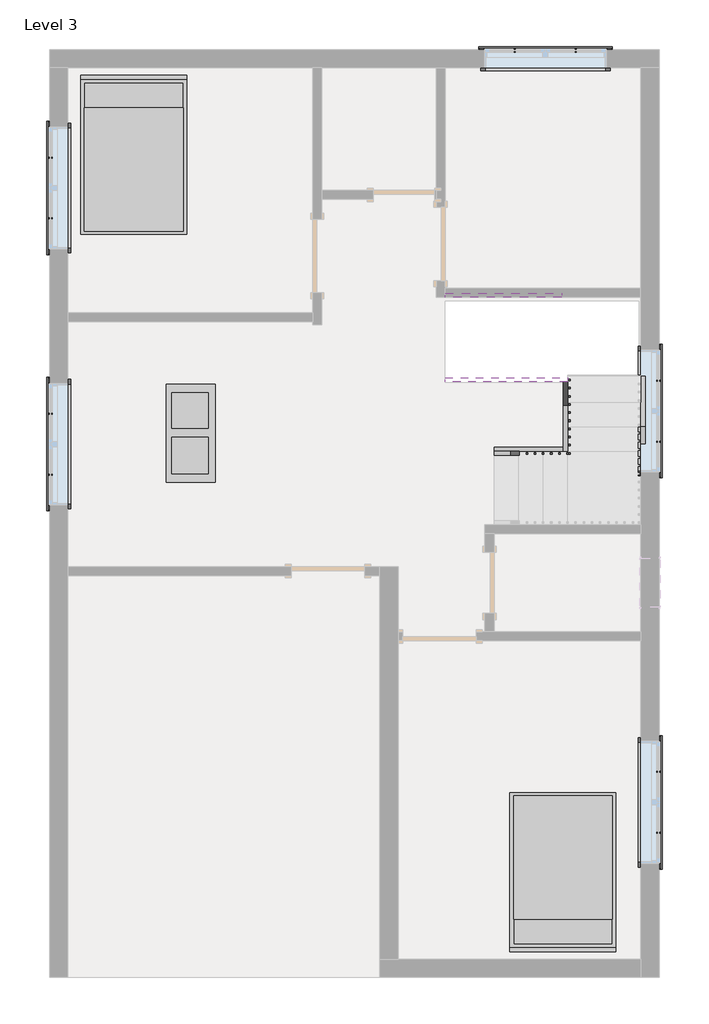
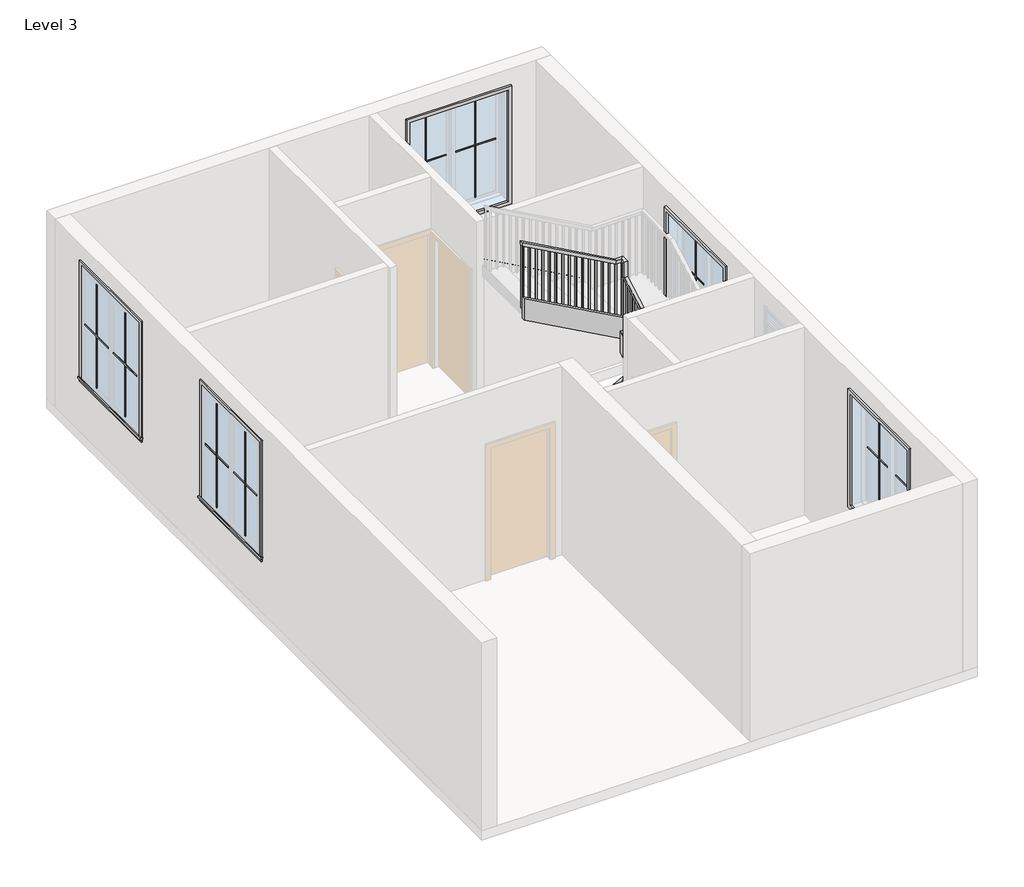
# One storey, part 2 of 2: 21 proxies, 6 members, 2 furniture elements, 1 railing.
"""IFC4 building model written with IfcOpenShell, lengths in millimetres."""

from ifc_helpers import new_model, si_unit, frame, origin, place, context, project, spatial, polyline, outline, extrude, faceted_brep, transform, mapped, element, save
from components import muntin_pattern_2x2_muntin_pattern_2x2_f6a80940, muntin_pattern_2x2_muntin_pattern_2x2_09b00a1c, trim_window_exterior_flat_with_sill_698ed857, trim_window_interior_flat_picture_frame_92551a5e, coffee_table_with_brass_mullions_11320_coffee_table_with_5962bef7, bed_17739_bed_17739_15c61121

model = new_model("IFC4")

# Units and contexts
model_context = context("Model", 3, world=origin())
ifc_project = project(units=[si_unit("LENGTHUNIT", "METRE", prefix="MILLI")], contexts=[model_context])

# Site, building, storey
site = spatial("IfcSite", under=ifc_project)
building = spatial("IfcBuilding", under=site)
storey = spatial("IfcBuildingStorey", under=building, Name="Level 3", Elevation=3200.4)

# Proxies
placement = place(None, origin())
muntin_pattern_2x2_muntin_pattern_2x2_shape = muntin_pattern_2x2_muntin_pattern_2x2_f6a80940(model_context)
element("IfcBuildingElementProxy", 1, Name="Muntin Pattern_2x2 : Muntin Pattern_2x2", ObjectType="Muntin Pattern_2x2 : Muntin Pattern_2x2", at=placement, inside=storey, context=model_context, shape_type="MappedRepresentation", body=[
    mapped(muntin_pattern_2x2_muntin_pattern_2x2_shape, transform((-4589.1575206, 441.8004493, 4184.65), x_axis=(0.0, 1.0, 0.0), y_axis=(-1.0, 0.0, 0.0), z_axis=(0.0, 0.0, 1.0))),
])
element("IfcBuildingElementProxy", 2, Name="Muntin Pattern_2x2 : Muntin Pattern_2x2", ObjectType="Muntin Pattern_2x2 : Muntin Pattern_2x2", at=placement, inside=storey, context=model_context, shape_type="MappedRepresentation", body=[
    mapped(muntin_pattern_2x2_muntin_pattern_2x2_shape, transform((-4589.1575206, 3632.6754493, 4184.65), x_axis=(0.0, 1.0, 0.0), y_axis=(-1.0, 0.0, 0.0), z_axis=(0.0, 0.0, 1.0))),
])
element("IfcBuildingElementProxy", 3, Name="Muntin Pattern_2x2 : Muntin Pattern_2x2", ObjectType="Muntin Pattern_2x2 : Muntin Pattern_2x2", at=placement, inside=storey, context=model_context, shape_type="MappedRepresentation", body=[
    mapped(muntin_pattern_2x2_muntin_pattern_2x2_shape, transform((1197.2799794, 5726.5879493, 4184.65), x_axis=(1.0, 0.0, 0.0), y_axis=(0.0, 1.0, 0.0), z_axis=(0.0, 0.0, 1.0))),
])
element("IfcBuildingElementProxy", 4, Name="Muntin Pattern_2x2 : Muntin Pattern_2x2", ObjectType="Muntin Pattern_2x2 : Muntin Pattern_2x2", at=placement, inside=storey, context=model_context, shape_type="MappedRepresentation", body=[
    mapped(muntin_pattern_2x2_muntin_pattern_2x2_shape, transform((2986.3924794, 1613.3754493, 4184.65), x_axis=(0.0, -1.0, 0.0), y_axis=(1.0, 0.0, 0.0), z_axis=(0.0, 0.0, 1.0))),
])
element("IfcBuildingElementProxy", 5, Name="Muntin Pattern_2x2 : Muntin Pattern_2x2", ObjectType="Muntin Pattern_2x2 : Muntin Pattern_2x2", at=placement, inside=storey, context=model_context, shape_type="MappedRepresentation", body=[
    mapped(muntin_pattern_2x2_muntin_pattern_2x2_shape, transform((2986.3924794, -3260.2495507, 4184.65), x_axis=(0.0, -1.0, 0.0), y_axis=(1.0, 0.0, 0.0), z_axis=(0.0, 0.0, 1.0))),
])
muntin_pattern_2x2_muntin_pattern_2x2_2_shape = muntin_pattern_2x2_muntin_pattern_2x2_09b00a1c(model_context)
element("IfcBuildingElementProxy", 6, Name="Muntin Pattern_2x2 : Muntin Pattern_2x2", ObjectType="Muntin Pattern_2x2 : Muntin Pattern_2x2", at=placement, inside=storey, context=model_context, shape_type="MappedRepresentation", body=[
    mapped(muntin_pattern_2x2_muntin_pattern_2x2_2_shape, transform((-4589.1575206, 1200.6254493, 4184.65), x_axis=(0.0, -1.0, 0.0), y_axis=(1.0, 0.0, 0.0), z_axis=(0.0, 0.0, 1.0))),
])
element("IfcBuildingElementProxy", 7, Name="Muntin Pattern_2x2 : Muntin Pattern_2x2", ObjectType="Muntin Pattern_2x2 : Muntin Pattern_2x2", at=placement, inside=storey, context=model_context, shape_type="MappedRepresentation", body=[
    mapped(muntin_pattern_2x2_muntin_pattern_2x2_2_shape, transform((-4589.1575206, 4391.5004493, 4184.65), x_axis=(0.0, -1.0, 0.0), y_axis=(1.0, 0.0, 0.0), z_axis=(0.0, 0.0, 1.0))),
])
element("IfcBuildingElementProxy", 8, Name="Muntin Pattern_2x2 : Muntin Pattern_2x2", ObjectType="Muntin Pattern_2x2 : Muntin Pattern_2x2", at=placement, inside=storey, context=model_context, shape_type="MappedRepresentation", body=[
    mapped(muntin_pattern_2x2_muntin_pattern_2x2_2_shape, transform((1956.1049794, 5726.5879493, 4184.65), x_axis=(-1.0, 0.0, 0.0), y_axis=(0.0, -1.0, 0.0), z_axis=(0.0, 0.0, 1.0))),
])
element("IfcBuildingElementProxy", 9, Name="Muntin Pattern_2x2 : Muntin Pattern_2x2", ObjectType="Muntin Pattern_2x2 : Muntin Pattern_2x2", at=placement, inside=storey, context=model_context, shape_type="MappedRepresentation", body=[
    mapped(muntin_pattern_2x2_muntin_pattern_2x2_2_shape, transform((2986.3924794, 854.5504493, 4184.65), x_axis=(0.0, 1.0, 0.0), y_axis=(-1.0, 0.0, 0.0), z_axis=(0.0, 0.0, 1.0))),
])
element("IfcBuildingElementProxy", 10, Name="Muntin Pattern_2x2 : Muntin Pattern_2x2", ObjectType="Muntin Pattern_2x2 : Muntin Pattern_2x2", at=placement, inside=storey, context=model_context, shape_type="MappedRepresentation", body=[
    mapped(muntin_pattern_2x2_muntin_pattern_2x2_2_shape, transform((2986.3924794, -4019.0745507, 4184.65), x_axis=(0.0, 1.0, 0.0), y_axis=(-1.0, 0.0, 0.0), z_axis=(0.0, 0.0, 1.0))),
])
trim_window_exterior_flat_with_sill_shape = trim_window_exterior_flat_with_sill_698ed857(model_context)
element("IfcBuildingElementProxy", 11, Name="Trim-Window-Exterior-Flat : with Sill", ObjectType="Trim-Window-Exterior-Flat : with Sill", at=placement, inside=storey, context=model_context, shape_type="MappedRepresentation", body=[
    mapped(trim_window_exterior_flat_with_sill_shape, transform((-4598.6825206, 821.2129493, 5943.6), x_axis=(0.0, -1.0, 0.0), y_axis=(0.0, 0.0, 1.0), z_axis=(-1.0, 0.0, 0.0))),
])
element("IfcBuildingElementProxy", 12, Name="Trim-Window-Exterior-Flat : with Sill", ObjectType="Trim-Window-Exterior-Flat : with Sill", at=placement, inside=storey, context=model_context, shape_type="MappedRepresentation", body=[
    mapped(trim_window_exterior_flat_with_sill_shape, transform((-4598.6825206, 4012.0879493, 5943.6), x_axis=(0.0, -1.0, 0.0), y_axis=(0.0, 0.0, 1.0), z_axis=(-1.0, 0.0, 0.0))),
])
element("IfcBuildingElementProxy", 13, Name="Trim-Window-Exterior-Flat : with Sill", ObjectType="Trim-Window-Exterior-Flat : with Sill", at=placement, inside=storey, context=model_context, shape_type="MappedRepresentation", body=[
    mapped(trim_window_exterior_flat_with_sill_shape, transform((1576.6924794, 5736.1129493, 5943.6), x_axis=(-1.0, 0.0, 0.0), y_axis=(0.0, 0.0, 1.0), z_axis=(0.0, 1.0, 0.0))),
])
element("IfcBuildingElementProxy", 14, Name="Trim-Window-Exterior-Flat : with Sill", ObjectType="Trim-Window-Exterior-Flat : with Sill", at=placement, inside=storey, context=model_context, shape_type="MappedRepresentation", body=[
    mapped(trim_window_exterior_flat_with_sill_shape, transform((2995.9174794, 1233.9629493, 5943.6), x_axis=(0.0, 1.0, 0.0), y_axis=(0.0, 0.0, 1.0), z_axis=(1.0, 0.0, 0.0))),
])
element("IfcBuildingElementProxy", 15, Name="Trim-Window-Exterior-Flat : with Sill", ObjectType="Trim-Window-Exterior-Flat : with Sill", at=placement, inside=storey, context=model_context, shape_type="MappedRepresentation", body=[
    mapped(trim_window_exterior_flat_with_sill_shape, transform((2995.9174794, -3639.6620507, 5943.6), x_axis=(0.0, 1.0, 0.0), y_axis=(0.0, 0.0, 1.0), z_axis=(1.0, 0.0, 0.0))),
])
trim_window_interior_flat_picture_frame_shape = trim_window_interior_flat_picture_frame_92551a5e(model_context)
element("IfcBuildingElementProxy", 16, Name="Trim-Window-Interior-Flat : Picture Frame", ObjectType="Trim-Window-Interior-Flat : Picture Frame", at=placement, inside=storey, context=model_context, shape_type="MappedRepresentation", body=[
    mapped(trim_window_interior_flat_picture_frame_shape, transform((-4370.0825206, 821.2129493, 5943.6), x_axis=(0.0, 1.0, 0.0), y_axis=(0.0, 0.0, 1.0), z_axis=(1.0, 0.0, 0.0))),
])
element("IfcBuildingElementProxy", 17, Name="Trim-Window-Interior-Flat : Picture Frame", ObjectType="Trim-Window-Interior-Flat : Picture Frame", at=placement, inside=storey, context=model_context, shape_type="MappedRepresentation", body=[
    mapped(trim_window_interior_flat_picture_frame_shape, transform((-4370.0825206, 4012.0879493, 5943.6), x_axis=(0.0, 1.0, 0.0), y_axis=(0.0, 0.0, 1.0), z_axis=(1.0, 0.0, 0.0))),
])
element("IfcBuildingElementProxy", 18, Name="Trim-Window-Interior-Flat : Picture Frame", ObjectType="Trim-Window-Interior-Flat : Picture Frame", at=placement, inside=storey, context=model_context, shape_type="MappedRepresentation", body=[
    mapped(trim_window_interior_flat_picture_frame_shape, transform((1576.6924794, 5507.5129493, 5943.6), x_axis=(1.0, 0.0, 0.0), y_axis=(0.0, 0.0, 1.0), z_axis=(0.0, -1.0, 0.0))),
])
element("IfcBuildingElementProxy", 19, Name="Trim-Window-Interior-Flat : Picture Frame", ObjectType="Trim-Window-Interior-Flat : Picture Frame", at=placement, inside=storey, context=model_context, shape_type="MappedRepresentation", body=[
    mapped(trim_window_interior_flat_picture_frame_shape, transform((2767.3174794, 1233.9629493, 5943.6), x_axis=(0.0, -1.0, 0.0), y_axis=(0.0, 0.0, 1.0), z_axis=(-1.0, 0.0, 0.0))),
])
element("IfcBuildingElementProxy", 20, Name="Trim-Window-Interior-Flat : Picture Frame", ObjectType="Trim-Window-Interior-Flat : Picture Frame", at=placement, inside=storey, context=model_context, shape_type="MappedRepresentation", body=[
    mapped(trim_window_interior_flat_picture_frame_shape, transform((2767.3174794, -3639.6620507, 5943.6), x_axis=(0.0, -1.0, 0.0), y_axis=(0.0, 0.0, 1.0), z_axis=(-1.0, 0.0, 0.0))),
])
coffee_table_with_brass_mullions_11320_coffee_table_with_shape = coffee_table_with_brass_mullions_11320_coffee_table_with_5962bef7(model_context)
element("IfcBuildingElementProxy", 21, Name="coffee_table_with_brass_mullions_11320 : coffee_table_with_brass_mullions_11320", ObjectType="coffee_table_with_brass_mullions_11320 : coffee_table_with_brass_mullions_11320", at=placement, inside=storey, context=model_context, shape_type="MappedRepresentation", body=[
    mapped(coffee_table_with_brass_mullions_11320_coffee_table_with_shape, transform((-2412.0418112, 1596.9678033, 3200.4), x_axis=(0.0, 1.0, 0.0), y_axis=(-1.0, 0.0, 0.0), z_axis=(0.0, 0.0, 1.0))),
])

# Furniture
bed_17739_bed_17739_shape = bed_17739_bed_17739_15c61121(model_context)
element("IfcFurniture", 22, ObjectType="Bed_17739 : Bed_17739", at=placement, inside=storey, context=model_context, shape_type="MappedRepresentation", body=[
    mapped(bed_17739_bed_17739_shape, transform((-3550.9325206, 4402.6129493, 3200.4), x_axis=(1.0, 0.0, 0.0), y_axis=(0.0, 1.0, 0.0), z_axis=(0.0, 0.0, 1.0))),
])
element("IfcFurniture", 23, ObjectType="Bed_17739 : Bed_17739", at=placement, inside=storey, context=model_context, shape_type="MappedRepresentation", body=[
    mapped(bed_17739_bed_17739_shape, transform((1795.7674794, -4487.3870507, 3200.4), x_axis=(-1.0, 0.0, 0.0), y_axis=(0.0, -1.0, 0.0), z_axis=(0.0, 0.0, 1.0))),
])

# Members
element("IfcMember", 24, ObjectType="Stringer - 2\" Width", at=placement, inside=storey, context=model_context, shape_type="SweptSolid", body=[
    extrude(outline(polyline([(3407.9983948, 938.5174794), (3200.4, 938.5174794), (3200.4, 1192.4619822), (3539.0974984, 1802.1174794), (3887.7761726, 1802.1174794), (3407.9983948, 938.5174794)])), frame((0.0, 732.3129493, 0.0), z_axis=(0.0, 1.0, 0.0), x_axis=(0.0, 0.0, 1.0)), (0.0, 0.0, 1.0), 50.8),
])
element("IfcMember", 25, ObjectType="Stringer - 2\" Width", at=placement, inside=storey, context=model_context, shape_type="SweptSolid", body=[
    extrude(outline(polyline([(732.3129493, 3736.653054), (732.3129493, 4085.3317281), (1595.9129493, 4565.1095059), (1595.9129493, 4216.4308318), (732.3129493, 3736.653054)])), frame((1802.1174794, 0.0, 0.0), z_axis=(1.0, 0.0, 0.0), x_axis=(0.0, 1.0, 0.0)), (0.0, 0.0, 1.0), 50.8),
])
element("IfcMember", 26, ObjectType="Stringer - 2\" Width", at=placement, inside=storey, context=model_context, shape_type="SweptSolid", body=[
    extrude(outline(polyline([(4413.9863873, 1852.9174794), (4762.6650614, 1852.9174794), (5609.3317281, 328.9174794), (5260.653054, 328.9174794), (4413.9863873, 1852.9174794)])), frame((0.0, 1595.9129493, 0.0), z_axis=(0.0, 1.0, 0.0), x_axis=(0.0, 0.0, 1.0)), (0.0, 0.0, 1.0), 50.8),
])
element("IfcMember", 27, ObjectType="Stringer - 2\" Width", at=placement, inside=storey, context=model_context, shape_type="SweptSolid", body=[
    extrude(outline(polyline([(3407.9983948, 938.5174794), (3200.4, 938.5174794), (3200.4, 1192.4619822), (3577.3317281, 1870.9390928), (3577.3317281, 1243.3174794), (3407.9983948, 938.5174794)])), frame((0.0, -232.8870507, 0.0), z_axis=(0.0, 1.0, 0.0), x_axis=(0.0, 0.0, 1.0)), (0.0, 0.0, 1.0), 50.8),
])
element("IfcMember", 28, ObjectType="Stringer - 2\" Width", at=placement, inside=storey, context=model_context, shape_type="SweptSolid", body=[
    extrude(outline(polyline([(714.2913359, 4075.3197207), (1037.1129493, 4254.6650614), (1664.7345627, 4254.6650614), (1341.9129493, 4075.3197207), (714.2913359, 4075.3197207)])), frame((2767.3174794, 0.0, 0.0), z_axis=(1.0, 0.0, 0.0), x_axis=(0.0, 1.0, 0.0)), (0.0, 0.0, 1.0), 50.8),
])
element("IfcMember", 29, ObjectType="Stringer - 2\" Width", at=placement, inside=storey, context=model_context, shape_type="SweptSolid", body=[
    extrude(outline(polyline([(4802.0419429, 1782.0390928), (5609.3317281, 328.9174794), (5260.653054, 328.9174794), (4802.0419429, 1154.4174794), (4802.0419429, 1782.0390928)])), frame((0.0, 2650.0129493, 0.0), z_axis=(0.0, 1.0, 0.0), x_axis=(0.0, 0.0, 1.0)), (0.0, 0.0, 1.0), 50.8),
])

# Railing
element("IfcRailing", 30, ObjectType="Handrail - Rectangular", at=placement, inside=storey, context=model_context, shape_type="SolidModel", body=[
    faceted_brep([(938.5174794, 732.3129493, 4284.1333333), (938.5174794, 732.3129493, 4226.020221), (938.5174794, 681.5129493, 4226.020221), (938.5174794, 681.5129493, 4284.1333333), (1776.7174794, 732.3129493, 4749.8), (1827.5174794, 732.3129493, 4719.9091099), (1827.5174794, 681.5129493, 4719.9091099), (1776.7174794, 681.5129493, 4749.8), (1776.7174794, 732.3129493, 5003.8), (1827.5174794, 732.3129493, 4953.0), (1827.5174794, 681.5129493, 4953.0), (1776.7174794, 681.5129493, 5003.8), (1852.9174794, 732.3129493, 5003.8), (1852.9174794, 732.3129493, 4953.0), (1903.7174794, 681.5129493, 4953.0), (1903.7174794, 681.5129493, 5003.8), (1852.9174794, 808.5129493, 5003.8), (1852.9174794, 821.6765516, 4953.0), (1903.7174794, 821.6765516, 4953.0), (1903.7174794, 808.5129493, 5003.8), (1852.9174794, 1570.5129493, 5427.1333333), (1852.9174794, 1621.3129493, 5397.2424432), (1903.7174794, 1621.3129493, 5397.2424432), (1903.7174794, 1570.5129493, 5427.1333333), (1852.9174794, 1570.5129493, 5681.1333333), (1852.9174794, 1621.3129493, 5630.3333333), (1903.7174794, 1621.3129493, 5630.3333333), (1903.7174794, 1570.5129493, 5681.1333333), (1852.9174794, 1646.7129493, 5681.1333333), (1852.9174794, 1646.7129493, 5630.3333333), (1903.7174794, 1697.5129493, 5630.3333333), (1903.7174794, 1697.5129493, 5681.1333333), (1776.7174794, 1646.7129493, 5681.1333333), (1763.5538772, 1646.7129493, 5630.3333333), (1763.5538772, 1697.5129493, 5630.3333333), (1776.7174794, 1697.5129493, 5681.1333333), (328.9174794, 1646.7129493, 6485.4666667), (328.9174794, 1697.5129493, 6485.4666667), (328.9174794, 1697.5129493, 6427.3535543), (328.9174794, 1646.7129493, 6427.3535543)], [[[0, 1, 2, 3]], [[1, 0, 4, 5]], [[2, 1, 5, 6]], [[3, 2, 6, 7]], [[0, 3, 7, 4]], [[5, 4, 8, 9]], [[6, 5, 9, 10]], [[7, 6, 10, 11]], [[4, 7, 11, 8]], [[9, 8, 12, 13]], [[10, 9, 13, 14]], [[11, 10, 14, 15]], [[8, 11, 15, 12]], [[13, 12, 16, 17]], [[14, 13, 17, 18]], [[15, 14, 18, 19]], [[12, 15, 19, 16]], [[17, 16, 20, 21]], [[18, 17, 21, 22]], [[19, 18, 22, 23]], [[16, 19, 23, 20]], [[21, 20, 24, 25]], [[22, 21, 25, 26]], [[23, 22, 26, 27]], [[20, 23, 27, 24]], [[25, 24, 28, 29]], [[26, 25, 29, 30]], [[27, 26, 30, 31]], [[24, 27, 31, 28]], [[29, 28, 32, 33]], [[30, 29, 33, 34]], [[31, 30, 34, 35]], [[28, 31, 35, 32]], [[36, 37, 38, 39]], [[33, 32, 36, 39]], [[34, 33, 39, 38]], [[35, 34, 38, 37]], [[32, 35, 37, 36]]]),
    extrude(outline(polyline([(6418.5341099, 344.7924794), (5401.7333333, 344.7924794), (5401.7333333, 363.8424794), (6407.9507765, 363.8424794), (6418.5341099, 344.7924794)])), frame((0.0, 1662.5879493, 0.0), z_axis=(0.0, 1.0, 0.0), x_axis=(0.0, 0.0, 1.0)), (0.0, 0.0, 1.0), 19.05),
    extrude(outline(polyline([(6362.0896654, 446.3924794), (5401.7333333, 446.3924794), (5401.7333333, 465.4424794), (6351.5063321, 465.4424794), (6362.0896654, 446.3924794)])), frame((0.0, 1662.5879493, 0.0), z_axis=(0.0, 1.0, 0.0), x_axis=(0.0, 0.0, 1.0)), (0.0, 0.0, 1.0), 19.05),
    extrude(outline(polyline([(6305.645221, 547.9924794), (5401.7333333, 547.9924794), (5401.7333333, 567.0424794), (6295.0618876, 567.0424794), (6305.645221, 547.9924794)])), frame((0.0, 1662.5879493, 0.0), z_axis=(0.0, 1.0, 0.0), x_axis=(0.0, 0.0, 1.0)), (0.0, 0.0, 1.0), 19.05),
    extrude(outline(polyline([(6249.2007765, 649.5924794), (5232.4, 649.5924794), (5232.4, 668.6424794), (6238.6174432, 668.6424794), (6249.2007765, 649.5924794)])), frame((0.0, 1662.5879493, 0.0), z_axis=(0.0, 1.0, 0.0), x_axis=(0.0, 0.0, 1.0)), (0.0, 0.0, 1.0), 19.05),
    extrude(outline(polyline([(6192.7563321, 751.1924794), (5232.4, 751.1924794), (5232.4, 770.2424794), (6182.1729988, 770.2424794), (6192.7563321, 751.1924794)])), frame((0.0, 1662.5879493, 0.0), z_axis=(0.0, 1.0, 0.0), x_axis=(0.0, 0.0, 1.0)), (0.0, 0.0, 1.0), 19.05),
    extrude(outline(polyline([(6136.3118876, 852.7924794), (5232.4, 852.7924794), (5232.4, 871.8424794), (6125.7285543, 871.8424794), (6136.3118876, 852.7924794)])), frame((0.0, 1662.5879493, 0.0), z_axis=(0.0, 1.0, 0.0), x_axis=(0.0, 0.0, 1.0)), (0.0, 0.0, 1.0), 19.05),
    extrude(outline(polyline([(6079.8674432, 954.3924794), (5063.0666667, 954.3924794), (5063.0666667, 973.4424794), (6069.2841099, 973.4424794), (6079.8674432, 954.3924794)])), frame((0.0, 1662.5879493, 0.0), z_axis=(0.0, 1.0, 0.0), x_axis=(0.0, 0.0, 1.0)), (0.0, 0.0, 1.0), 19.05),
    extrude(outline(polyline([(6023.4229988, 1055.9924794), (5063.0666667, 1055.9924794), (5063.0666667, 1075.0424794), (6012.8396654, 1075.0424794), (6023.4229988, 1055.9924794)])), frame((0.0, 1662.5879493, 0.0), z_axis=(0.0, 1.0, 0.0), x_axis=(0.0, 0.0, 1.0)), (0.0, 0.0, 1.0), 19.05),
    extrude(outline(polyline([(5966.9785543, 1157.5924794), (5063.0666667, 1157.5924794), (5063.0666667, 1176.6424794), (5956.395221, 1176.6424794), (5966.9785543, 1157.5924794)])), frame((0.0, 1662.5879493, 0.0), z_axis=(0.0, 1.0, 0.0), x_axis=(0.0, 0.0, 1.0)), (0.0, 0.0, 1.0), 19.05),
    extrude(outline(polyline([(5910.5341099, 1259.1924794), (4893.7333333, 1259.1924794), (4893.7333333, 1278.2424794), (5899.9507765, 1278.2424794), (5910.5341099, 1259.1924794)])), frame((0.0, 1662.5879493, 0.0), z_axis=(0.0, 1.0, 0.0), x_axis=(0.0, 0.0, 1.0)), (0.0, 0.0, 1.0), 19.05),
    extrude(outline(polyline([(5854.0896654, 1360.7924794), (4893.7333333, 1360.7924794), (4893.7333333, 1379.8424794), (5843.5063321, 1379.8424794), (5854.0896654, 1360.7924794)])), frame((0.0, 1662.5879493, 0.0), z_axis=(0.0, 1.0, 0.0), x_axis=(0.0, 0.0, 1.0)), (0.0, 0.0, 1.0), 19.05),
    extrude(outline(polyline([(5797.645221, 1462.3924794), (4893.7333333, 1462.3924794), (4893.7333333, 1481.4424794), (5787.0618876, 1481.4424794), (5797.645221, 1462.3924794)])), frame((0.0, 1662.5879493, 0.0), z_axis=(0.0, 1.0, 0.0), x_axis=(0.0, 0.0, 1.0)), (0.0, 0.0, 1.0), 19.05),
    extrude(outline(polyline([(5741.2007765, 1563.9924794), (4724.4, 1563.9924794), (4724.4, 1583.0424794), (5730.6174432, 1583.0424794), (5741.2007765, 1563.9924794)])), frame((0.0, 1662.5879493, 0.0), z_axis=(0.0, 1.0, 0.0), x_axis=(0.0, 0.0, 1.0)), (0.0, 0.0, 1.0), 19.05),
    extrude(outline(polyline([(5684.7563321, 1665.5924794), (4724.4, 1665.5924794), (4724.4, 1684.6424794), (5674.1729988, 1684.6424794), (5684.7563321, 1665.5924794)])), frame((0.0, 1662.5879493, 0.0), z_axis=(0.0, 1.0, 0.0), x_axis=(0.0, 0.0, 1.0)), (0.0, 0.0, 1.0), 19.05),
    extrude(outline(polyline([(5628.3118876, 1767.1924794), (4724.4, 1767.1924794), (4724.4, 1786.2424794), (5617.7285543, 1786.2424794), (5628.3118876, 1767.1924794)])), frame((0.0, 1662.5879493, 0.0), z_axis=(0.0, 1.0, 0.0), x_axis=(0.0, 0.0, 1.0)), (0.0, 0.0, 1.0), 19.05),
    extrude(outline(polyline([(1868.7924794, 1611.7879493), (1868.7924794, 1630.8379493), (1887.8424794, 1630.8379493), (1887.8424794, 1611.7879493), (1868.7924794, 1611.7879493)])), frame((0.0, 0.0, 4385.7333333), z_axis=(0.0, 0.0, 1.0), x_axis=(1.0, 0.0, 0.0)), (0.0, 0.0, 1.0), 1244.6),
    extrude(outline(polyline([(1529.2379493, 5346.0896654), (1529.2379493, 4385.7333333), (1510.1879493, 4385.7333333), (1510.1879493, 5335.5063321), (1529.2379493, 5346.0896654)])), frame((1868.7924794, 0.0, 0.0), z_axis=(1.0, 0.0, 0.0), x_axis=(0.0, 1.0, 0.0)), (0.0, 0.0, 1.0), 19.05),
    extrude(outline(polyline([(1427.6379493, 5289.645221), (1427.6379493, 4385.7333333), (1408.5879493, 4385.7333333), (1408.5879493, 5279.0618876), (1427.6379493, 5289.645221)])), frame((1868.7924794, 0.0, 0.0), z_axis=(1.0, 0.0, 0.0), x_axis=(0.0, 1.0, 0.0)), (0.0, 0.0, 1.0), 19.05),
    extrude(outline(polyline([(1326.0379493, 5233.2007765), (1326.0379493, 4216.4), (1306.9879493, 4216.4), (1306.9879493, 5222.6174432), (1326.0379493, 5233.2007765)])), frame((1868.7924794, 0.0, 0.0), z_axis=(1.0, 0.0, 0.0), x_axis=(0.0, 1.0, 0.0)), (0.0, 0.0, 1.0), 19.05),
    extrude(outline(polyline([(1224.4379493, 5176.7563321), (1224.4379493, 4216.4), (1205.3879493, 4216.4), (1205.3879493, 5166.1729988), (1224.4379493, 5176.7563321)])), frame((1868.7924794, 0.0, 0.0), z_axis=(1.0, 0.0, 0.0), x_axis=(0.0, 1.0, 0.0)), (0.0, 0.0, 1.0), 19.05),
    extrude(outline(polyline([(1122.8379493, 5120.3118876), (1122.8379493, 4216.4), (1103.7879493, 4216.4), (1103.7879493, 5109.7285543), (1122.8379493, 5120.3118876)])), frame((1868.7924794, 0.0, 0.0), z_axis=(1.0, 0.0, 0.0), x_axis=(0.0, 1.0, 0.0)), (0.0, 0.0, 1.0), 19.05),
    extrude(outline(polyline([(1021.2379493, 5063.8674432), (1021.2379493, 4047.0666667), (1002.1879493, 4047.0666667), (1002.1879493, 5053.2841099), (1021.2379493, 5063.8674432)])), frame((1868.7924794, 0.0, 0.0), z_axis=(1.0, 0.0, 0.0), x_axis=(0.0, 1.0, 0.0)), (0.0, 0.0, 1.0), 19.05),
    extrude(outline(polyline([(919.6379493, 5007.4229988), (919.6379493, 4047.0666667), (900.5879493, 4047.0666667), (900.5879493, 4996.8396654), (919.6379493, 5007.4229988)])), frame((1868.7924794, 0.0, 0.0), z_axis=(1.0, 0.0, 0.0), x_axis=(0.0, 1.0, 0.0)), (0.0, 0.0, 1.0), 19.05),
    extrude(outline(polyline([(818.0379493, 4950.9785543), (818.0379493, 4047.0666667), (798.9879493, 4047.0666667), (798.9879493, 4940.395221), (818.0379493, 4950.9785543)])), frame((1868.7924794, 0.0, 0.0), z_axis=(1.0, 0.0, 0.0), x_axis=(0.0, 1.0, 0.0)), (0.0, 0.0, 1.0), 19.05),
    extrude(outline(polyline([(1843.3924794, 716.4379493), (1862.4424794, 716.4379493), (1862.4424794, 697.3879493), (1843.3924794, 697.3879493), (1843.3924794, 716.4379493)])), frame((0.0, 0.0, 3877.7333333), z_axis=(0.0, 0.0, 1.0), x_axis=(1.0, 0.0, 0.0)), (0.0, 0.0, 1.0), 1075.2666667),
    extrude(outline(polyline([(4672.2841099, 1741.7924794), (3708.4, 1741.7924794), (3708.4, 1760.8424794), (4682.8674432, 1760.8424794), (4672.2841099, 1741.7924794)])), frame((0.0, 697.3879493, 0.0), z_axis=(0.0, 1.0, 0.0), x_axis=(0.0, 0.0, 1.0)), (0.0, 0.0, 1.0), 19.05),
    extrude(outline(polyline([(4615.8396654, 1640.1924794), (3708.4, 1640.1924794), (3708.4, 1659.2424794), (4626.4229988, 1659.2424794), (4615.8396654, 1640.1924794)])), frame((0.0, 697.3879493, 0.0), z_axis=(0.0, 1.0, 0.0), x_axis=(0.0, 0.0, 1.0)), (0.0, 0.0, 1.0), 19.05),
    extrude(outline(polyline([(4559.395221, 1538.5924794), (3708.4, 1538.5924794), (3708.4, 1557.6424794), (4569.9785543, 1557.6424794), (4559.395221, 1538.5924794)])), frame((0.0, 697.3879493, 0.0), z_axis=(0.0, 1.0, 0.0), x_axis=(0.0, 0.0, 1.0)), (0.0, 0.0, 1.0), 19.05),
    extrude(outline(polyline([(4502.9507765, 1436.9924794), (3539.0666667, 1436.9924794), (3539.0666667, 1456.0424794), (4513.5341099, 1456.0424794), (4502.9507765, 1436.9924794)])), frame((0.0, 697.3879493, 0.0), z_axis=(0.0, 1.0, 0.0), x_axis=(0.0, 0.0, 1.0)), (0.0, 0.0, 1.0), 19.05),
    extrude(outline(polyline([(4446.5063321, 1335.3924794), (3539.0666667, 1335.3924794), (3539.0666667, 1354.4424794), (4457.0896654, 1354.4424794), (4446.5063321, 1335.3924794)])), frame((0.0, 697.3879493, 0.0), z_axis=(0.0, 1.0, 0.0), x_axis=(0.0, 0.0, 1.0)), (0.0, 0.0, 1.0), 19.05),
    extrude(outline(polyline([(4390.0618876, 1233.7924794), (3539.0666667, 1233.7924794), (3539.0666667, 1252.8424794), (4400.645221, 1252.8424794), (4390.0618876, 1233.7924794)])), frame((0.0, 697.3879493, 0.0), z_axis=(0.0, 1.0, 0.0), x_axis=(0.0, 0.0, 1.0)), (0.0, 0.0, 1.0), 19.05),
    extrude(outline(polyline([(4333.6174432, 1132.1924794), (3369.7333333, 1132.1924794), (3369.7333333, 1151.2424794), (4344.2007765, 1151.2424794), (4333.6174432, 1132.1924794)])), frame((0.0, 697.3879493, 0.0), z_axis=(0.0, 1.0, 0.0), x_axis=(0.0, 0.0, 1.0)), (0.0, 0.0, 1.0), 19.05),
    extrude(outline(polyline([(4277.1729988, 1030.5924794), (3369.7333333, 1030.5924794), (3369.7333333, 1049.6424794), (4287.7563321, 1049.6424794), (4277.1729988, 1030.5924794)])), frame((0.0, 697.3879493, 0.0), z_axis=(0.0, 1.0, 0.0), x_axis=(0.0, 0.0, 1.0)), (0.0, 0.0, 1.0), 19.05),
    extrude(outline(polyline([(1868.7924794, 1662.5879493), (1868.7924794, 1681.6379493), (1887.8424794, 1681.6379493), (1887.8424794, 1662.5879493), (1868.7924794, 1662.5879493)])), frame((0.0, 0.0, 4555.0666667), z_axis=(0.0, 0.0, 1.0), x_axis=(1.0, 0.0, 0.0)), (0.0, 0.0, 1.0), 1075.2666667),
    extrude(outline(polyline([(1868.7924794, 716.4379493), (1887.8424794, 716.4379493), (1887.8424794, 697.3879493), (1868.7924794, 697.3879493), (1868.7924794, 716.4379493)])), frame((0.0, 0.0, 3877.7333333), z_axis=(0.0, 0.0, 1.0), x_axis=(1.0, 0.0, 0.0)), (0.0, 0.0, 1.0), 1075.2666667),
    extrude(outline(polyline([(6427.3535543, 328.9174794), (5401.7333333, 328.9174794), (5401.7333333, 347.9674794), (6416.770221, 347.9674794), (6427.3535543, 328.9174794)])), frame((0.0, 1662.5879493, 0.0), z_axis=(0.0, 1.0, 0.0), x_axis=(0.0, 0.0, 1.0)), (0.0, 0.0, 1.0), 19.05),
    extrude(outline(polyline([(4226.020221, 938.5174794), (3369.7333333, 938.5174794), (3369.7333333, 957.5674794), (4236.6035543, 957.5674794), (4226.020221, 938.5174794)])), frame((0.0, 697.3879493, 0.0), z_axis=(0.0, 1.0, 0.0), x_axis=(0.0, 0.0, 1.0)), (0.0, 0.0, 1.0), 19.05),
])

save(model, "model.ifc")

# Revit data of these elements
# Type "Muntin Pattern_2x2 : Muntin Pattern_2x2"
#   Width [instance default] = 4' - 0"
#   Thickness = 0' - 0 1/2"
#   Height [instance default] = 4' - 0"
#   Distance = 0' - 0 3/4"
#   Interior Material [instance default] = none
#   Exterior Material [instance default] = none
#   Default Elevation = 0
# Type "Trim-Window-Exterior-Flat : with Sill"
#   Trim Width = 0' - 2 1/4"
#   Trim Thickness_Picture Frame = 0' - 1 1/4"
#   Trim Thickness_with Sill = 0' - 0 3/4"
#   Sill Thickness = 0' - 1 1/4"
#   Opening Width [instance default] = 2' - 0"
#   Opening Height [instance default] = 3' - 0"
#   Default Elevation = 4' - 0"
#   Sill = yes
#   Picture Frame = no
#   Trim Material [instance default] = none
# Type "Trim-Window-Interior-Flat : Picture Frame"
#   Trim Thickness_Picture Frame = 0' - 1 1/4"
#   Trim Width = 0' - 2 1/4"
#   Trim Thickness_with Sill = 0' - 0 3/4"
#   Sill Thickness = 0' - 1 1/4"
#   Opening Width [instance default] = 2' - 0"
#   Opening Height [instance default] = 3' - 0"
#   Default Elevation = 4' - 0"
#   Sill = no
#   Picture Frame = yes
#   Trim Material [instance default] = none
# Type "coffee_table_with_brass_mullions_11320 : coffee_table_with_brass_mullions_11320"
#   Default Elevation = 0
# Type "Bed_17739 : Bed_17739"
#   Default Elevation = 0
# Type "Handrail - Rectangular"
#   Assembly Code = "C2010400"
#   built-in parameter 1008612 = 0.0416667 (stored number, unit not read)
#   built-in parameter 1008611 = 0.0416667 (stored number, unit not read)
#   built-in parameter 1008609 = 0.333333 (stored number, unit not read)
#   built-in parameter 1008604 = 0.166667 (stored number, unit not read)
#   built-in parameter 1008603 = 0.166667 (stored number, unit not read)
#   Railing Height = 3' - 0"
#   built-in parameter 1008630 = 2
#   built-in parameter 1008610 = 2
#   built-in parameter 1008618 = Baluster - Square : 3/4"
# Elements 1, 2, 3, 4, 5, 6, 7, 8, 9, 10 (IfcBuildingElementProxy, "Muntin Pattern_2x2 : Muntin Pattern_2x2")
#   Width = 2' - 0 5/8"
#   Height = 5' - 6 1/2"
#   Interior Material = Wood - Stained
#   Exterior Material = Clad - White
#   Phase Created = New Construction
#   Materials on its faces: "Clad - White", "Wood - Stained"
# Elements 11, 12, 13, 14, 15 (IfcBuildingElementProxy, "Trim-Window-Exterior-Flat : with Sill")
#   Opening Width = 5' - 0"
#   Opening Height = 6' - 0"
#   Trim Material = Clad - White
#   Phase Created = New Construction
#   Materials on its faces: "Clad - White"
# Elements 16, 17, 18, 19, 20 (IfcBuildingElementProxy, "Trim-Window-Interior-Flat : Picture Frame")
#   Opening Width = 5' - 0"
#   Opening Height = 6' - 0"
#   Trim Material = Wood - Stained
#   Phase Created = New Construction
#   Materials on its faces: "Wood - Stained"
# Element 21 (IfcBuildingElementProxy, "coffee_table_with_brass_mullions_11320 : coffee_table_with_brass_mullions_11320")
#   Phase Created = New Construction
#   Materials on its faces: "Default Wall", "TABLE", "Glass", "Default"
# Elements 22, 23 (IfcFurniture, "Bed_17739 : Bed_17739")
#   Phase Created = New Construction
#   Materials on its faces: "legs", "sheets", "bed frame", "Blanket"
# Elements 24, 25, 26, 27, 28, 29 (IfcMember, "Stringer - 2\" Width")
#   Phase Created = New Construction
# Element 30 (IfcRailing, "Handrail - Rectangular")
#   Phase Created = New Construction
# Materials
#   "Clad - White": class "Wood", colour RGB 242 242 238, transparency 0, Cost = 0
#   "Wood - Stained": class "Wood", colour RGB 224 178 126, transparency 0, Cost = 0
#   "Default Wall": colour RGB 128 128 128, transparency 0, Cost = 0
#   "TABLE": class "Generic", colour RGB 120 120 120, transparency 0, Cost = 0
#   "Glass": class "Glass", colour RGB 0 128 192, transparency 0.75, Description = "Soda Lime Glass", Cost = 0
#   "Default": colour RGB 127 127 127, transparency 0, Cost = 0
#   "legs": colour RGB 90 73 37, transparency 0, Cost = 0
#   "sheets": colour RGB 200 195 176, transparency 0, Cost = 0
#   "bed frame": colour RGB 90 73 37, transparency 0, Cost = 0
#   "Blanket": class "System", colour RGB 59 0 1, transparency 0, Cost = 0
